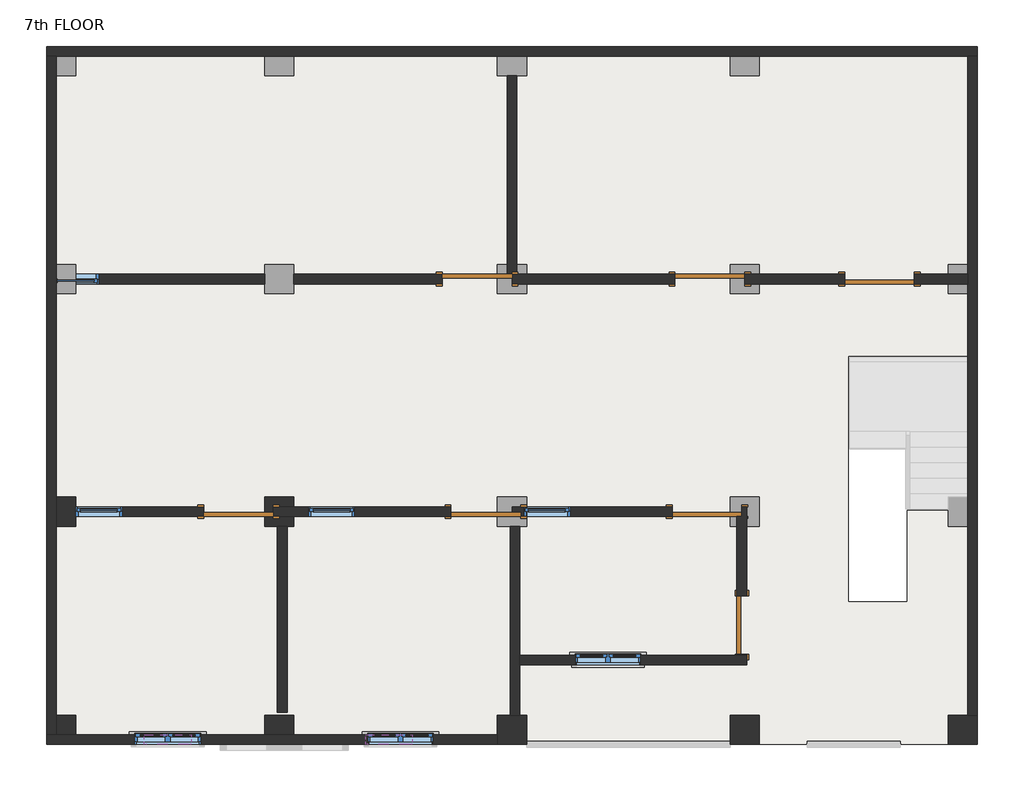
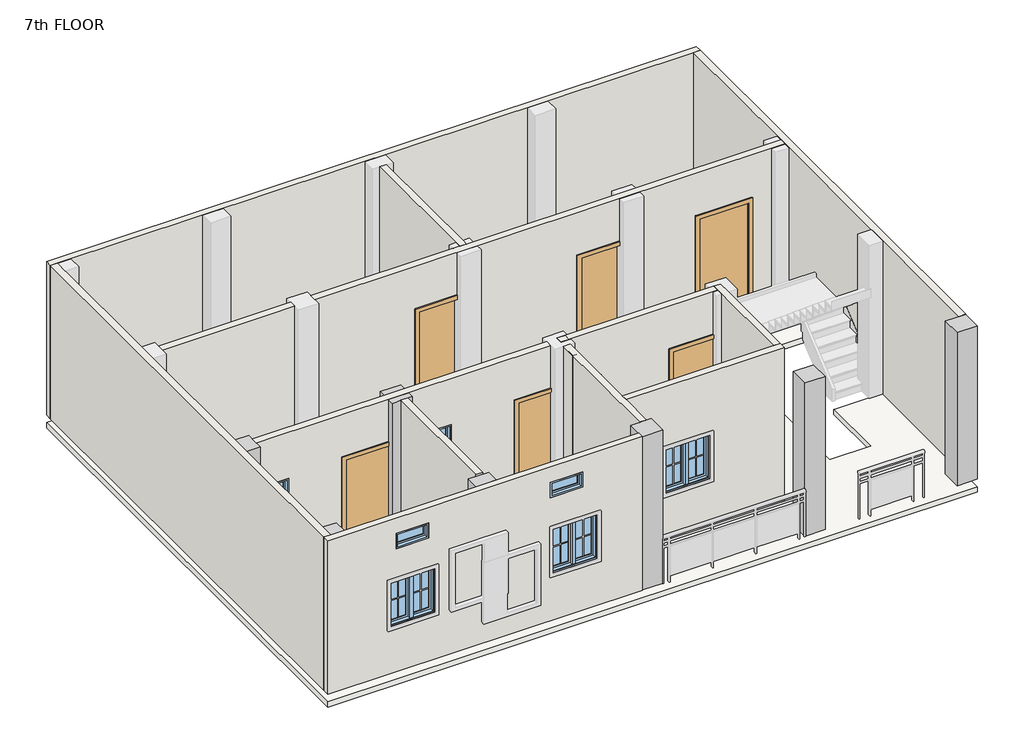
# One storey, part 1 of 2: 15 walls, 9 windows, 7 columns, 7 doors, 1 slab.
"""IFC4 building model written with IfcOpenShell, lengths in millimetres."""

from ifc_helpers import new_model, si_unit, frame, origin, place, context, project, spatial, polyline, outline, extrude, faceted_brep, transform, mapped, element, save
from components import door_e00f436c, door_a1797ceb, window_4c2727af, window_0bf3737e, window_78893e6c, window_0d9958e7

model = new_model("IFC4")

# Units and contexts
model_context = context("Model", 3, world=origin())
ifc_project = project(units=[si_unit("LENGTHUNIT", "METRE", prefix="MILLI")], contexts=[model_context])

# Site, building, storey
site = spatial("IfcSite", under=ifc_project)
building = spatial("IfcBuilding", under=site)
storey = spatial("IfcBuildingStorey", under=building, Name="7th FLOOR", Elevation=21183.6)

# Columns
placement = place(None, origin())
element("IfcColumn", 1, ObjectType="column family : column family", at=placement, inside=storey, context=model_context, shape_type="Brep", body=[
    faceted_brep([(-12576.097125, 2486.2065522, 21188.6), (-12957.097125, 2486.2065522, 21188.6), (-12957.097125, 2867.2065522, 21188.6), (-12576.097125, 2867.2065522, 21188.6), (-12576.097125, 2740.2065522, 21188.6), (-12842.797125, 2740.2065522, 21188.6), (-12842.797125, 2613.2065522, 21188.6), (-12576.097125, 2613.2065522, 21188.6), (-12576.097125, 2486.2065522, 24226.6), (-12576.097125, 2613.2065522, 24226.6), (-12957.097125, 2486.2065522, 24226.6), (-12957.097125, 2613.2065522, 24226.6), (-12957.097125, 2613.2065522, 23317.2), (-12957.097125, 2740.2065522, 23317.2), (-12957.097125, 2740.2065522, 24226.6), (-12957.097125, 2867.2065522, 24226.6), (-12576.097125, 2867.2065522, 24226.6), (-12842.797125, 2613.2065522, 23317.2), (-12842.797125, 2740.2065522, 23317.2), (-12576.097125, 2740.2065522, 24226.6)], [[[0, 1, 2, 3, 4, 5, 6, 7]], [[8, 0, 7, 9]], [[1, 0, 8, 10]], [[2, 1, 10, 11, 12, 13, 14, 15]], [[3, 2, 15, 16]], [[10, 8, 9, 11]], [[6, 17, 12, 11, 9, 7]], [[13, 18, 5, 4, 19, 14]], [[3, 16, 19, 4]], [[16, 15, 14, 19]], [[17, 18, 13, 12]], [[18, 17, 6, 5]]]),
])
element("IfcColumn", 2, ObjectType="column family : column family", at=placement, inside=storey, context=model_context, shape_type="SweptSolid", body=[
    extrude(outline(polyline([(-15433.597125, 2867.2065522), (-15433.597125, 2486.2065522), (-15687.597125, 2486.2065522), (-15687.597125, 2867.2065522), (-15433.597125, 2867.2065522)])), frame((0.0, 0.0, 21188.6), z_axis=(0.0, 0.0, 1.0), x_axis=(1.0, 0.0, 0.0)), (0.0, 0.0, 1.0), 3038.0),
])
element("IfcColumn", 3, ObjectType="column family : column family", at=placement, inside=storey, context=model_context, shape_type="SweptSolid", body=[
    extrude(outline(polyline([(-15433.597125, 9.7065522), (-15433.597125, -244.2934478), (-15687.597125, -244.2934478), (-15687.597125, 9.7065522), (-15433.597125, 9.7065522)])), frame((0.0, 0.0, 21188.6), z_axis=(0.0, 0.0, 1.0), x_axis=(1.0, 0.0, 0.0)), (0.0, 0.0, 1.0), 3038.0),
])
element("IfcColumn", 4, ObjectType="column family : column family", at=placement, inside=storey, context=model_context, shape_type="SweptSolid", body=[
    extrude(outline(polyline([(-3622.597125, 9.7065522), (-3622.597125, -371.2934478), (-4003.597125, -371.2934478), (-4003.597125, 9.7065522), (-3622.597125, 9.7065522)])), frame((0.0, 0.0, 21188.6), z_axis=(0.0, 0.0, 1.0), x_axis=(1.0, 0.0, 0.0)), (0.0, 0.0, 1.0), 3038.0),
])
element("IfcColumn", 5, ObjectType="column family : column family", at=placement, inside=storey, context=model_context, shape_type="SweptSolid", body=[
    extrude(outline(polyline([(-6480.097125, 9.7065522), (-6480.097125, -371.2934478), (-6861.097125, -371.2934478), (-6861.097125, 9.7065522), (-6480.097125, 9.7065522)])), frame((0.0, 0.0, 21188.6), z_axis=(0.0, 0.0, 1.0), x_axis=(1.0, 0.0, 0.0)), (0.0, 0.0, 1.0), 3038.0),
])
element("IfcColumn", 6, ObjectType="column family : column family", at=placement, inside=storey, context=model_context, shape_type="SweptSolid", body=[
    extrude(outline(polyline([(-9528.097125, 9.7065522), (-9528.097125, -371.2934478), (-9909.097125, -371.2934478), (-9909.097125, 9.7065522), (-9528.097125, 9.7065522)])), frame((0.0, 0.0, 21188.6), z_axis=(0.0, 0.0, 1.0), x_axis=(1.0, 0.0, 0.0)), (0.0, 0.0, 1.0), 3038.0),
])
element("IfcColumn", 7, ObjectType="column family : column family", at=placement, inside=storey, context=model_context, shape_type="SweptSolid", body=[
    extrude(outline(polyline([(-12957.097125, 9.7065522), (-12576.097125, 9.7065522), (-12576.097125, -244.2934478), (-12957.097125, -244.2934478), (-12957.097125, 9.7065522)])), frame((0.0, 0.0, 21188.6), z_axis=(0.0, 0.0, 1.0), x_axis=(1.0, 0.0, 0.0)), (0.0, 0.0, 1.0), 3038.0),
])

# Doors
door_shape = door_e00f436c(model_context)
element("IfcDoor", 8, ObjectType="Single-Flush : 30\" x 80\"", at=placement, inside=storey, context=model_context, shape_type="MappedRepresentation", body=[
    mapped(door_shape, transform((-6708.697125, 1190.8065522, 21183.6), x_axis=(0.0, -1.0, 0.0), y_axis=(1.0, 0.0, 0.0), z_axis=(0.0, 0.0, 1.0))),
])
door_2_shape = door_a1797ceb(model_context)
element("IfcDoor", 9, ObjectType="Single-Flush : 36\" x 84\"", at=placement, inside=storey, context=model_context, shape_type="MappedRepresentation", body=[
    mapped(door_2_shape, transform((-10175.797125, 5724.7065522, 21183.6), x_axis=(1.0, 0.0, 0.0), y_axis=(0.0, 1.0, 0.0), z_axis=(0.0, 0.0, 1.0))),
])
element("IfcDoor", 10, ObjectType="Single-Flush : 36\" x 84\"", at=placement, inside=storey, context=model_context, shape_type="MappedRepresentation", body=[
    mapped(door_2_shape, transform((-10061.497125, 2676.7065522, 21183.6), x_axis=(-1.0, 0.0, 0.0), y_axis=(0.0, -1.0, 0.0), z_axis=(0.0, 0.0, 1.0))),
])
element("IfcDoor", 11, ObjectType="Single-Flush : 36\" x 84\"", at=placement, inside=storey, context=model_context, shape_type="MappedRepresentation", body=[
    mapped(door_2_shape, transform((-13299.997125, 2676.7065522, 21183.6), x_axis=(-1.0, 0.0, 0.0), y_axis=(0.0, -1.0, 0.0), z_axis=(0.0, 0.0, 1.0))),
])
element("IfcDoor", 12, ObjectType="Single-Flush : 36\" x 84\"", at=placement, inside=storey, context=model_context, shape_type="MappedRepresentation", body=[
    mapped(door_2_shape, transform((-7127.797125, 5724.7065522, 21183.6), x_axis=(1.0, 0.0, 0.0), y_axis=(0.0, 1.0, 0.0), z_axis=(0.0, 0.0, 1.0))),
])
element("IfcDoor", 13, ObjectType="Single-Flush : 36\" x 84\"", at=placement, inside=storey, context=model_context, shape_type="MappedRepresentation", body=[
    mapped(door_2_shape, transform((-7165.897125, 2676.7065522, 21183.6), x_axis=(-1.0, 0.0, 0.0), y_axis=(0.0, -1.0, 0.0), z_axis=(0.0, 0.0, 1.0))),
])
element("IfcDoor", 14, ObjectType="Single-Flush : 36\" x 84\"", at=placement, inside=storey, context=model_context, shape_type="MappedRepresentation", body=[
    mapped(door_2_shape, transform((-4905.297125, 5724.7065522, 21183.6), x_axis=(-1.0, 0.0, 0.0), y_axis=(0.0, -1.0, 0.0), z_axis=(0.0, 0.0, 1.0))),
])

# Slab
element("IfcSlab", 15, ObjectType="Generic - 4\"", at=placement, inside=storey, context=model_context, shape_type="SweptSolid", body=[
    extrude(outline(polyline([(-3622.597125, 8772.7065522), (-3622.597125, -371.2934478), (-15814.597125, -371.2934478), (-15814.597125, 8772.7065522), (-3622.597125, 8772.7065522)]), holes=[polyline([(-3734.357125, 4711.0719226), (-5310.2646464, 4711.0719226), (-5310.2646464, 1502.3126957), (-4547.7736682, 1502.3126957), (-4547.7736682, 2699.911213), (-3734.357125, 2699.911213), (-3734.357125, 4711.0719226)])]), frame((0.0, 0.0, 20929.6), z_axis=(0.0, 0.0, 1.0), x_axis=(1.0, 0.0, 0.0)), (0.0, 0.0, 1.0), 101.6),
])

# Walls
element("IfcWall", 16, ObjectType="Generic - 5\"", at=placement, inside=storey, context=model_context, shape_type="Brep", body=[
    faceted_brep([(-15814.597125, 8645.7065522, 21183.6), (-15687.597125, 8645.7065522, 21183.6), (-3749.597125, 8645.7065522, 21183.6), (-3622.597125, 8645.7065522, 21183.6), (-3622.597125, 8645.7065522, 24231.6), (-3749.597125, 8645.7065522, 24231.6), (-15687.597125, 8645.7065522, 24231.6), (-15814.597125, 8645.7065522, 24231.6), (-15814.597125, 8772.7065522, 21183.6), (-15814.597125, 8772.7065522, 24231.6), (-3622.597125, 8772.7065522, 24231.6), (-3622.597125, 8772.7065522, 21183.6)], [[[0, 1, 2, 3, 4, 5, 6, 7]], [[8, 9, 10, 11]], [[3, 2, 1, 0, 8, 11]], [[7, 6, 5, 4, 10, 9]], [[4, 3, 11, 10]], [[0, 7, 9, 8]]]),
])
element("IfcWall", 17, ObjectType="Generic - 5\"", at=placement, inside=storey, context=model_context, shape_type="Brep", body=[
    faceted_brep([(-3749.597125, 8645.7065522, 21183.6), (-3749.597125, 5788.2065522, 21183.6), (-3749.597125, 5661.2065522, 21183.6), (-3749.597125, 9.7065522, 21183.6), (-3749.597125, 9.7065522, 24231.6), (-3749.597125, 5661.2065522, 24231.6), (-3749.597125, 5788.2065522, 24231.6), (-3749.597125, 8645.7065522, 24231.6), (-3622.597125, 8645.7065522, 21183.6), (-3622.597125, 8645.7065522, 24231.6), (-3622.597125, 9.7065522, 24231.6), (-3622.597125, 9.7065522, 24226.6), (-3622.597125, 9.7065522, 21188.6), (-3622.597125, 9.7065522, 21183.6)], [[[0, 1, 2, 3, 4, 5, 6, 7]], [[8, 9, 10, 11, 12, 13]], [[3, 2, 1, 0, 8, 13]], [[4, 3, 13, 12, 11, 10]], [[7, 6, 5, 4, 10, 9]], [[0, 7, 9, 8]]]),
])
element("IfcWall", 18, ObjectType="Generic - 5\"", at=placement, inside=storey, context=model_context, shape_type="Brep", body=[
    faceted_brep([(-9909.097125, -244.2934478, 21183.6), (-15687.597125, -244.2934478, 21183.6), (-15814.597125, -244.2934478, 21183.6), (-15814.597125, -244.2934478, 24231.6), (-15687.597125, -244.2934478, 24231.6), (-9909.097125, -244.2934478, 24231.6), (-13795.297125, -244.2934478, 23012.4), (-14658.897125, -244.2934478, 23012.4), (-14658.897125, -244.2934478, 22098.0), (-13795.297125, -244.2934478, 22098.0), (-10747.297125, -244.2934478, 23012.4), (-11610.897125, -244.2934478, 23012.4), (-11610.897125, -244.2934478, 22098.0), (-10747.297125, -244.2934478, 22098.0), (-13922.297125, -244.2934478, 23926.8), (-14531.897125, -244.2934478, 23926.8), (-14531.897125, -244.2934478, 23622.0), (-13922.297125, -244.2934478, 23622.0), (-11026.697125, -244.2934478, 23926.8), (-11636.297125, -244.2934478, 23926.8), (-11636.297125, -244.2934478, 23622.0), (-11026.697125, -244.2934478, 23622.0), (-9909.097125, -371.2934478, 21183.6), (-9909.097125, -371.2934478, 21188.6), (-9909.097125, -371.2934478, 24226.6), (-9909.097125, -371.2934478, 24231.6), (-15814.597125, -371.2934478, 24231.6), (-15814.597125, -371.2934478, 21183.6), (-13795.297125, -371.2934478, 23012.4), (-13795.297125, -371.2934478, 22098.0), (-14658.897125, -371.2934478, 22098.0), (-14658.897125, -371.2934478, 23012.4), (-10747.297125, -371.2934478, 23012.4), (-10747.297125, -371.2934478, 22098.0), (-11610.897125, -371.2934478, 22098.0), (-11610.897125, -371.2934478, 23012.4), (-13922.297125, -371.2934478, 23926.8), (-13922.297125, -371.2934478, 23622.0), (-14531.897125, -371.2934478, 23622.0), (-14531.897125, -371.2934478, 23926.8), (-11026.697125, -371.2934478, 23926.8), (-11026.697125, -371.2934478, 23622.0), (-11636.297125, -371.2934478, 23622.0), (-11636.297125, -371.2934478, 23926.8)], [[[0, 1, 2, 3, 4, 5], [6, 7, 8, 9], [10, 11, 12, 13], [14, 15, 16, 17], [18, 19, 20, 21]], [[22, 23, 24, 25, 26, 27], [28, 29, 30, 31], [32, 33, 34, 35], [36, 37, 38, 39], [40, 41, 42, 43]], [[2, 1, 0, 22, 27]], [[5, 4, 3, 26, 25]], [[0, 5, 25, 24, 23, 22]], [[3, 2, 27, 26]], [[29, 28, 6, 9]], [[30, 29, 9, 8]], [[31, 30, 8, 7]], [[28, 31, 7, 6]], [[33, 32, 10, 13]], [[34, 33, 13, 12]], [[35, 34, 12, 11]], [[32, 35, 11, 10]], [[37, 36, 14, 17]], [[38, 37, 17, 16]], [[39, 38, 16, 15]], [[36, 39, 15, 14]], [[41, 40, 18, 21]], [[42, 41, 21, 20]], [[43, 42, 20, 19]], [[40, 43, 19, 18]]]),
])
element("IfcWall", 19, ObjectType="Generic - 5\"", at=placement, inside=storey, context=model_context, shape_type="Brep", body=[
    faceted_brep([(-15687.597125, -244.2934478, 21183.6), (-15687.597125, 8645.7065522, 21183.6), (-15687.597125, 8645.7065522, 21188.6), (-15687.597125, 8645.7065522, 24226.6), (-15687.597125, 8645.7065522, 24231.6), (-15687.597125, -244.2934478, 24231.6), (-15687.597125, -244.2934478, 24226.6), (-15687.597125, -244.2934478, 21188.6), (-15814.597125, -244.2934478, 21183.6), (-15814.597125, -244.2934478, 24231.6), (-15814.597125, 8645.7065522, 24231.6), (-15814.597125, 8645.7065522, 21183.6)], [[[0, 1, 2, 3, 4, 5, 6, 7]], [[8, 9, 10, 11]], [[1, 0, 8, 11]], [[5, 4, 10, 9]], [[4, 3, 2, 1, 11, 10]], [[0, 7, 6, 5, 9, 8]]]),
])
element("IfcWall", 20, ObjectType="Generic - 5\"", at=placement, inside=storey, context=model_context, shape_type="SweptSolid", body=[
    extrude(outline(polyline([(21183.6, -15433.597125), (21183.6, -12957.097125), (24231.6, -12957.097125), (24231.6, -15433.597125), (23317.2, -15433.597125), (23317.2, -15128.797125), (21488.4, -15128.797125), (21488.4, -15433.597125), (21183.6, -15433.597125)])), frame((0.0, 5661.2065522, 0.0), z_axis=(0.0, 1.0, 0.0), x_axis=(0.0, 0.0, 1.0)), (0.0, 0.0, 1.0), 127.0),
])
element("IfcWall", 21, ObjectType="Generic - 5\"", at=placement, inside=storey, context=model_context, shape_type="Brep", body=[
    faceted_brep([(-9782.097125, 8391.7065522, 21183.6), (-9782.097125, 5788.2065522, 21183.6), (-9782.097125, 5788.2065522, 21188.6), (-9782.097125, 5788.2065522, 23317.2), (-9782.097125, 5788.2065522, 24226.6), (-9782.097125, 5788.2065522, 24231.6), (-9782.097125, 8391.7065522, 24231.6), (-9655.097125, 8391.7065522, 21183.6), (-9655.097125, 8391.7065522, 24231.6), (-9655.097125, 5788.2065522, 24231.6), (-9655.097125, 5788.2065522, 24226.6), (-9655.097125, 5788.2065522, 21188.6), (-9655.097125, 5788.2065522, 21183.6), (-9718.597125, 5788.2065522, 21183.6)], [[[0, 1, 2, 3, 4, 5, 6]], [[7, 8, 9, 10, 11, 12]], [[1, 0, 7, 12, 13]], [[6, 5, 9, 8]], [[0, 6, 8, 7]], [[5, 4, 3, 2, 1, 13, 12, 11, 10, 9]]]),
])
element("IfcWall", 22, ObjectType="Generic - 5\"", at=placement, inside=storey, context=model_context, shape_type="Brep", body=[
    faceted_brep([(-6670.597125, 5661.2065522, 21183.6), (-5362.497125, 5661.2065522, 21183.6), (-5362.497125, 5661.2065522, 23317.2), (-4448.097125, 5661.2065522, 23317.2), (-4448.097125, 5661.2065522, 21183.6), (-3749.597125, 5661.2065522, 21183.6), (-3749.597125, 5661.2065522, 21188.6), (-3749.597125, 5661.2065522, 24226.6), (-3749.597125, 5661.2065522, 24231.6), (-12576.097125, 5661.2065522, 24231.6), (-12576.097125, 5661.2065522, 21183.6), (-10632.997125, 5661.2065522, 21183.6), (-10632.997125, 5661.2065522, 23317.2), (-9909.097125, 5661.2065522, 23317.2), (-9718.597125, 5661.2065522, 23317.2), (-9718.597125, 5661.2065522, 21188.6), (-9718.597125, 5661.2065522, 21183.6), (-7584.997125, 5661.2065522, 21183.6), (-7584.997125, 5661.2065522, 23317.2), (-6861.097125, 5661.2065522, 23317.2), (-6670.597125, 5661.2065522, 23317.2), (-6670.597125, 5661.2065522, 21188.6), (-5362.497125, 5788.2065522, 23317.2), (-5362.497125, 5788.2065522, 21183.6), (-6670.597125, 5788.2065522, 21183.6), (-6670.597125, 5788.2065522, 21188.6), (-6670.597125, 5788.2065522, 23317.2), (-6861.097125, 5788.2065522, 23317.2), (-7584.997125, 5788.2065522, 23317.2), (-7584.997125, 5788.2065522, 21183.6), (-9655.097125, 5788.2065522, 21183.6), (-9718.597125, 5788.2065522, 21183.6), (-9718.597125, 5788.2065522, 21188.6), (-9718.597125, 5788.2065522, 23317.2), (-9782.097125, 5788.2065522, 23317.2), (-9909.097125, 5788.2065522, 23317.2), (-10632.997125, 5788.2065522, 23317.2), (-10632.997125, 5788.2065522, 21183.6), (-12576.097125, 5788.2065522, 21183.6), (-12576.097125, 5788.2065522, 24231.6), (-9782.097125, 5788.2065522, 24231.6), (-9655.097125, 5788.2065522, 24231.6), (-3749.597125, 5788.2065522, 24231.6), (-3749.597125, 5788.2065522, 24226.6), (-3749.597125, 5788.2065522, 21188.6), (-3749.597125, 5788.2065522, 21183.6), (-4448.097125, 5788.2065522, 21183.6), (-4448.097125, 5788.2065522, 23317.2)], [[[0, 1, 2, 3, 4, 5, 6, 7, 8, 9, 10, 11, 12, 13, 14, 15, 16, 17, 18, 19, 20, 21]], [[22, 23, 24, 25, 26, 27, 28, 29, 30, 31, 32, 33, 34, 35, 36, 37, 38, 39, 40, 41, 42, 43, 44, 45, 46, 47]], [[11, 10, 38, 37]], [[17, 16, 31, 30, 29]], [[46, 45, 5, 4]], [[24, 23, 1, 0]], [[9, 8, 42, 41, 40, 39]], [[10, 9, 39, 38]], [[8, 7, 6, 5, 45, 44, 43, 42]], [[33, 32, 31, 16, 15, 14]], [[36, 35, 34, 33, 14, 13, 12]], [[37, 36, 12, 11]], [[26, 25, 24, 0, 21, 20]], [[28, 27, 26, 20, 19, 18]], [[29, 28, 18, 17]], [[2, 1, 23, 22]], [[3, 2, 22, 47]], [[4, 3, 47, 46]]]),
])
element("IfcWall", 23, ObjectType="Generic - 5\"", at=placement, inside=storey, context=model_context, shape_type="Brep", body=[
    faceted_brep([(-14823.997125, 2613.2065522, 21488.4), (-15433.597125, 2613.2065522, 21488.4), (-15433.597125, 2613.2065522, 21183.6), (-13757.197125, 2613.2065522, 21183.6), (-13757.197125, 2613.2065522, 23317.2), (-12957.097125, 2613.2065522, 23317.2), (-12842.797125, 2613.2065522, 23317.2), (-12842.797125, 2613.2065522, 21188.6), (-12842.797125, 2613.2065522, 21183.6), (-10518.697125, 2613.2065522, 21183.6), (-10518.697125, 2613.2065522, 23317.2), (-9909.097125, 2613.2065522, 23317.2), (-9909.097125, 2613.2065522, 24231.6), (-15433.597125, 2613.2065522, 24231.6), (-15433.597125, 2613.2065522, 23317.2), (-14823.997125, 2613.2065522, 23317.2), (-12385.597125, 2613.2065522, 23317.2), (-11775.997125, 2613.2065522, 23317.2), (-11775.997125, 2613.2065522, 21488.4), (-12385.597125, 2613.2065522, 21488.4), (-15433.597125, 2740.2065522, 21183.6), (-15433.597125, 2740.2065522, 21488.4), (-14823.997125, 2740.2065522, 21488.4), (-14823.997125, 2740.2065522, 23317.2), (-15433.597125, 2740.2065522, 23317.2), (-15433.597125, 2740.2065522, 24231.6), (-9909.097125, 2740.2065522, 24231.6), (-9909.097125, 2740.2065522, 23317.2), (-10518.697125, 2740.2065522, 23317.2), (-10518.697125, 2740.2065522, 21183.6), (-12842.797125, 2740.2065522, 21183.6), (-12842.797125, 2740.2065522, 21188.6), (-12842.797125, 2740.2065522, 23317.2), (-12957.097125, 2740.2065522, 23317.2), (-13757.197125, 2740.2065522, 23317.2), (-13757.197125, 2740.2065522, 21183.6), (-12385.597125, 2740.2065522, 23317.2), (-12385.597125, 2740.2065522, 21488.4), (-11775.997125, 2740.2065522, 21488.4), (-11775.997125, 2740.2065522, 23317.2)], [[[0, 1, 2, 3, 4, 5, 6, 7, 8, 9, 10, 11, 12, 13, 14, 15], [16, 17, 18, 19]], [[20, 21, 22, 23, 24, 25, 26, 27, 28, 29, 30, 31, 32, 33, 34, 35], [36, 37, 38, 39]], [[30, 29, 9, 8]], [[20, 35, 3, 2]], [[26, 12, 11, 27]], [[13, 12, 26, 25]], [[14, 13, 25, 24]], [[2, 1, 21, 20]], [[28, 10, 9, 29]], [[10, 28, 27, 11]], [[4, 3, 35, 34]], [[6, 5, 4, 34, 33, 32]], [[8, 7, 6, 32, 31, 30]], [[22, 21, 1, 0]], [[23, 22, 0, 15]], [[24, 23, 15, 14]], [[37, 36, 16, 19]], [[38, 37, 19, 18]], [[39, 38, 18, 17]], [[36, 39, 17, 16]]]),
])
element("IfcWall", 24, ObjectType="Generic - 5\"", at=placement, inside=storey, context=model_context, shape_type="Brep", body=[
    faceted_brep([(-9616.997125, 9.7065522, 21183.6), (-9616.997125, 670.1065522, 21183.6), (-9616.997125, 797.1065522, 21183.6), (-9616.997125, 2486.2065522, 21183.6), (-9616.997125, 2486.2065522, 24231.6), (-9616.997125, 797.1065522, 24231.6), (-9616.997125, 670.1065522, 24231.6), (-9616.997125, 9.7065522, 24231.6), (-9743.997125, 9.7065522, 21183.6), (-9743.997125, 9.7065522, 24231.6), (-9743.997125, 2486.2065522, 24231.6), (-9743.997125, 2486.2065522, 21183.6)], [[[0, 1, 2, 3, 4, 5, 6, 7]], [[8, 9, 10, 11]], [[3, 2, 1, 0, 8, 11]], [[4, 3, 11, 10]], [[7, 6, 5, 4, 10, 9]], [[0, 7, 9, 8]]]),
])
element("IfcWall", 25, ObjectType="Generic - 5\"", at=placement, inside=storey, context=model_context, shape_type="SweptSolid", body=[
    extrude(outline(polyline([(-9743.997125, 2181.4065522), (-9743.997125, 2486.2065522), (-9616.997125, 2486.2065522), (-9616.997125, 2181.4065522), (-9743.997125, 2181.4065522)])), frame((0.0, 0.0, 21183.6), z_axis=(0.0, 0.0, 1.0), x_axis=(1.0, 0.0, 0.0)), (0.0, 0.0, 1.0), 3048.0),
])
element("IfcWall", 26, ObjectType="Generic - 5\"", at=placement, inside=storey, context=model_context, shape_type="Brep", body=[
    faceted_brep([(-6772.197125, 2613.2065522, 24231.6), (-9718.597125, 2613.2065522, 24231.6), (-9718.597125, 2613.2065522, 24226.6), (-9718.597125, 2613.2065522, 21188.6), (-9718.597125, 2613.2065522, 21183.6), (-7623.097125, 2613.2065522, 21183.6), (-7623.097125, 2613.2065522, 23317.2), (-6861.097125, 2613.2065522, 23317.2), (-6772.197125, 2613.2065522, 23317.2), (-6772.197125, 2613.2065522, 24226.6), (-9566.197125, 2613.2065522, 23317.2), (-9528.097125, 2613.2065522, 23317.2), (-8956.597125, 2613.2065522, 23317.2), (-8956.597125, 2613.2065522, 21488.4), (-9528.097125, 2613.2065522, 21488.4), (-9566.197125, 2613.2065522, 21488.4), (-9718.597125, 2740.2065522, 24231.6), (-6772.197125, 2740.2065522, 24231.6), (-6772.197125, 2740.2065522, 23317.2), (-6861.097125, 2740.2065522, 23317.2), (-7623.097125, 2740.2065522, 23317.2), (-7623.097125, 2740.2065522, 21183.6), (-9718.597125, 2740.2065522, 21183.6), (-9718.597125, 2740.2065522, 21188.6), (-9718.597125, 2740.2065522, 24226.6), (-9566.197125, 2740.2065522, 23317.2), (-9566.197125, 2740.2065522, 21488.4), (-9528.097125, 2740.2065522, 21488.4), (-8956.597125, 2740.2065522, 21488.4), (-8956.597125, 2740.2065522, 23317.2), (-9528.097125, 2740.2065522, 23317.2)], [[[0, 1, 2, 3, 4, 5, 6, 7, 8, 9], [10, 11, 12, 13, 14, 15]], [[16, 17, 18, 19, 20, 21, 22, 23, 24], [25, 26, 27, 28, 29, 30]], [[4, 22, 21, 5]], [[1, 0, 17, 16]], [[4, 3, 2, 1, 16, 24, 23, 22]], [[26, 25, 10, 15]], [[28, 27, 26, 15, 14, 13]], [[29, 28, 13, 12]], [[25, 30, 29, 12, 11, 10]], [[20, 6, 5, 21]], [[6, 20, 19, 18, 8, 7]], [[17, 0, 9, 8, 18]]]),
])
element("IfcWall", 27, ObjectType="Generic - 5\"", at=placement, inside=storey, context=model_context, shape_type="Brep", body=[
    faceted_brep([(-6645.197125, 797.1065522, 21183.6), (-6645.197125, 809.8065522, 21183.6), (-6645.197125, 809.8065522, 23215.6), (-6645.197125, 1571.8065522, 23215.6), (-6645.197125, 1571.8065522, 21183.6), (-6645.197125, 2740.2065522, 21183.6), (-6645.197125, 2740.2065522, 21188.6), (-6645.197125, 2740.2065522, 24226.6), (-6645.197125, 2740.2065522, 24231.6), (-6645.197125, 797.1065522, 24231.6), (-6772.197125, 809.8065522, 23215.6), (-6772.197125, 809.8065522, 21183.6), (-6772.197125, 797.1065522, 21183.6), (-6772.197125, 797.1065522, 24231.6), (-6772.197125, 2613.2065522, 24231.6), (-6772.197125, 2740.2065522, 24231.6), (-6772.197125, 2740.2065522, 23317.2), (-6772.197125, 2613.2065522, 23317.2), (-6772.197125, 2613.2065522, 21188.6), (-6772.197125, 2613.2065522, 21183.6), (-6772.197125, 1571.8065522, 21183.6), (-6772.197125, 1571.8065522, 23215.6), (-6708.697125, 2613.2065522, 21183.6), (-6708.697125, 2740.2065522, 21183.6), (-6708.697125, 2613.2065522, 23317.2), (-6708.697125, 2613.2065522, 21188.6), (-6708.697125, 2740.2065522, 23317.2), (-6708.697125, 2740.2065522, 21188.6)], [[[0, 1, 2, 3, 4, 5, 6, 7, 8, 9]], [[10, 11, 12, 13, 14, 15, 16, 17, 18, 19, 20, 21]], [[20, 19, 22, 23, 5, 4]], [[12, 11, 1, 0]], [[9, 8, 15, 14, 13]], [[24, 25, 22, 19, 18, 17]], [[26, 24, 17, 16]], [[22, 25, 24, 26, 27, 23]], [[8, 7, 6, 5, 23, 27, 26, 16, 15]], [[0, 9, 13, 12]], [[2, 1, 11, 10]], [[3, 2, 10, 21]], [[4, 3, 21, 20]]]),
])
element("IfcWall", 28, ObjectType="Generic - 5\"", at=placement, inside=storey, context=model_context, shape_type="Brep", body=[
    faceted_brep([(-9718.597125, 2613.2065522, 21183.6), (-9566.197125, 2613.2065522, 21183.6), (-9566.197125, 2613.2065522, 21488.4), (-9566.197125, 2613.2065522, 23317.2), (-9566.197125, 2613.2065522, 24231.6), (-9718.597125, 2613.2065522, 24231.6), (-9718.597125, 2613.2065522, 24226.6), (-9718.597125, 2613.2065522, 21188.6), (-9718.597125, 2740.2065522, 21183.6), (-9718.597125, 2740.2065522, 21188.6), (-9718.597125, 2740.2065522, 24226.6), (-9718.597125, 2740.2065522, 24231.6), (-9566.197125, 2740.2065522, 24231.6), (-9566.197125, 2740.2065522, 23317.2), (-9566.197125, 2740.2065522, 21488.4), (-9566.197125, 2740.2065522, 21183.6)], [[[0, 1, 2, 3, 4, 5, 6, 7]], [[8, 9, 10, 11, 12, 13, 14, 15]], [[1, 0, 8, 15]], [[4, 3, 2, 1, 15, 14, 13, 12]], [[5, 4, 12, 11]], [[0, 7, 6, 5, 11, 10, 9, 8]]]),
])
element("IfcWall", 29, ObjectType="Generic - 5\"", at=placement, inside=storey, context=model_context, shape_type="SweptSolid", body=[
    extrude(outline(polyline([(-12791.997125, 47.8065522), (-12791.997125, 2486.2065522), (-12664.997125, 2486.2065522), (-12664.997125, 47.8065522), (-12791.997125, 47.8065522)])), frame((0.0, 0.0, 21183.6), z_axis=(0.0, 0.0, 1.0), x_axis=(1.0, 0.0, 0.0)), (0.0, 0.0, 1.0), 3048.0),
])
element("IfcWall", 30, ObjectType="Generic - 5\"", at=placement, inside=storey, context=model_context, shape_type="Brep", body=[
    faceted_brep([(-9616.997125, 670.1065522, 21183.6), (-6645.197125, 670.1065522, 21183.6), (-6645.197125, 670.1065522, 24231.6), (-9616.997125, 670.1065522, 24231.6), (-8029.497125, 670.1065522, 23012.4), (-8029.497125, 670.1065522, 22098.0), (-8893.097125, 670.1065522, 22098.0), (-8893.097125, 670.1065522, 23012.4), (-9616.997125, 797.1065522, 21183.6), (-9616.997125, 797.1065522, 24231.6), (-6772.197125, 797.1065522, 24231.6), (-6645.197125, 797.1065522, 24231.6), (-6645.197125, 797.1065522, 21183.6), (-6772.197125, 797.1065522, 21183.6), (-8029.497125, 797.1065522, 23012.4), (-8893.097125, 797.1065522, 23012.4), (-8893.097125, 797.1065522, 22098.0), (-8029.497125, 797.1065522, 22098.0)], [[[0, 1, 2, 3], [4, 5, 6, 7]], [[8, 9, 10, 11, 12, 13], [14, 15, 16, 17]], [[1, 0, 8, 13, 12]], [[3, 2, 11, 10, 9]], [[0, 3, 9, 8]], [[2, 1, 12, 11]], [[5, 4, 14, 17]], [[6, 5, 17, 16]], [[7, 6, 16, 15]], [[4, 7, 15, 14]]]),
])

# Windows
window_shape = window_4c2727af(model_context)
element("IfcWindow", 31, ObjectType="Fixed : 24\" x 12\"", at=placement, inside=storey, context=model_context, shape_type="MappedRepresentation", body=[
    mapped(window_shape, transform((-14188.997125, -307.7934478, 22707.6), x_axis=(1.0, 0.0, 0.0), y_axis=(0.0, 1.0, 0.0), z_axis=(0.0, 0.0, 1.0))),
])
element("IfcWindow", 32, ObjectType="Fixed : 24\" x 12\"", at=placement, inside=storey, context=model_context, shape_type="MappedRepresentation", body=[
    mapped(window_shape, transform((-11293.397125, -307.7934478, 22707.6), x_axis=(1.0, 0.0, 0.0), y_axis=(0.0, 1.0, 0.0), z_axis=(0.0, 0.0, 1.0))),
])
window_2_shape = window_0bf3737e(model_context)
element("IfcWindow", 33, ObjectType="Fixed : 24\" x 72\"", at=placement, inside=storey, context=model_context, shape_type="MappedRepresentation", body=[
    mapped(window_2_shape, transform((-15471.697125, 5724.7065522, 21183.6), x_axis=(-1.0, 0.0, 0.0), y_axis=(0.0, -1.0, 0.0), z_axis=(0.0, 0.0, 1.0))),
])
window_3_shape = window_78893e6c(model_context)
element("IfcWindow", 34, ObjectType="Fixed : 24\" x 72\"", at=placement, inside=storey, context=model_context, shape_type="MappedRepresentation", body=[
    mapped(window_3_shape, transform((-15166.897125, 2676.7065522, 21183.6), x_axis=(-1.0, 0.0, 0.0), y_axis=(0.0, -1.0, 0.0), z_axis=(0.0, 0.0, 1.0))),
])
element("IfcWindow", 35, ObjectType="Fixed : 24\" x 72\"", at=placement, inside=storey, context=model_context, shape_type="MappedRepresentation", body=[
    mapped(window_3_shape, transform((-12118.897125, 2676.7065522, 21183.6), x_axis=(-1.0, 0.0, 0.0), y_axis=(0.0, -1.0, 0.0), z_axis=(0.0, 0.0, 1.0))),
])
element("IfcWindow", 36, ObjectType="Fixed : 24\" x 72\"", at=placement, inside=storey, context=model_context, shape_type="MappedRepresentation", body=[
    mapped(window_3_shape, transform((-9299.497125, 2676.7065522, 21183.6), x_axis=(-1.0, 0.0, 0.0), y_axis=(0.0, -1.0, 0.0), z_axis=(0.0, 0.0, 1.0))),
])
window_4_shape = window_0d9958e7(model_context)
element("IfcWindow", 37, ObjectType="Window-Casement-Double : 34\" x 36\"", at=placement, inside=storey, context=model_context, shape_type="MappedRepresentation", body=[
    mapped(window_4_shape, transform((-14227.097125, -307.7934478, 21183.6), x_axis=(1.0, 0.0, 0.0), y_axis=(0.0, 1.0, 0.0), z_axis=(0.0, 0.0, 1.0))),
])
element("IfcWindow", 38, ObjectType="Window-Casement-Double : 34\" x 36\"", at=placement, inside=storey, context=model_context, shape_type="MappedRepresentation", body=[
    mapped(window_4_shape, transform((-11179.097125, -307.7934478, 21183.6), x_axis=(1.0, 0.0, 0.0), y_axis=(0.0, 1.0, 0.0), z_axis=(0.0, 0.0, 1.0))),
])
element("IfcWindow", 39, ObjectType="Window-Casement-Double : 34\" x 36\"", at=placement, inside=storey, context=model_context, shape_type="MappedRepresentation", body=[
    mapped(window_4_shape, transform((-8461.297125, 733.6065522, 21183.6), x_axis=(1.0, 0.0, 0.0), y_axis=(0.0, 1.0, 0.0), z_axis=(0.0, 0.0, 1.0))),
])

save(model, "model.ifc")

# Revit data of these elements
# Type "column family : column family"
#   w2 [instance default] = 0' - 9.88189"
#   w1 [instance default] = 0' - 9.01575"
#   Depth = 1' - 11.62205"
#   Width = 1' - 11.62205"
# Type "Single-Flush : 30\" x 80\""
#   Type Mark = "5"
#   Construction Type Id = "MDOOR"
#   Assembly Code = "C1020"
#   Analytic Construction = "Metal"
#   Thickness = 0' - 2"
#   Heat Transfer Coefficient (U) = 0.651978 BTU/(h·ft²·°F)
#   Height = 6' - 8"
#   Trim Projection Ext = 0' - 1"
#   Trim Projection Int = 0' - 1"
#   Trim Width = 0' - 3"
#   Width = 2' - 6"
#   Define Thermal Properties by = 1
#   Define Thermal Properties by = 1
#   Door Material = Door - Panel
#   Frame Material = Door - Frame
#   Visual Light Transmittance = 0
#   Solar Heat Gain Coefficient = 0
#   Function = (empty or 0)
#   Wall Closure = (empty or 0)
# Type "Single-Flush : 36\" x 84\""
#   Type Mark = "1"
#   Construction Type Id = "MDOOR"
#   Assembly Code = "C1020"
#   Analytic Construction = "Metal"
#   Thickness = 0' - 2"
#   Heat Transfer Coefficient (U) = 0.651978 BTU/(h·ft²·°F)
#   Height = 7' - 0"
#   Trim Projection Ext = 0' - 1"
#   Trim Projection Int = 0' - 1"
#   Trim Width = 0' - 3"
#   Width = 3' - 0"
#   Define Thermal Properties by = 1
#   Define Thermal Properties by = 1
#   Door Material = Door - Panel
#   Frame Material = Door - Frame
#   Visual Light Transmittance = 0
#   Solar Heat Gain Coefficient = 0
#   Function = (empty or 0)
#   Wall Closure = (empty or 0)
# Type "Generic - 4\""
#   Assembly Code = "B1010"
#   Function = 0
#   Layers, outside or top first: 0' - 4" no material (function 1)
# Type "Generic - 5\""
#   Assembly Code = "B2010"
#   Layers, outside or top first: 0' - 5" no material (function 1)
# Type "Fixed : 24\" x 12\""
#   Type Mark = "4"
#   Construction Type Id = "GSP4R"
#   Assembly Code = "B2020100"
#   Analytic Construction = "1/8 in Pilkington single glazing"
#   Visual Light Transmittance = 0.9
#   Solar Heat Gain Coefficient = 0.78
#   Heat Transfer Coefficient (U) = 0.6496 BTU/(h·ft²·°F)
#   Height = 1' - 0"
#   Default Sill Height = 3' - 0"
#   Width = 2' - 0"
#   Window Inset = 0' - 0 3/4"
#   Define Thermal Properties by = 1
#   Define Thermal Properties by = 1
#   Glass Pane Material = Glass
#   Sash Material = Sash
#   Wall Closure = (empty or 0)
# Type "Fixed : 24\" x 72\""
#   Type Mark = "7"
#   Construction Type Id = "GSP4R"
#   Assembly Code = "B2020100"
#   Analytic Construction = "1/8 in Pilkington single glazing"
#   Visual Light Transmittance = 0.9
#   Solar Heat Gain Coefficient = 0.78
#   Heat Transfer Coefficient (U) = 0.6496 BTU/(h·ft²·°F)
#   Height = 6' - 0"
#   Default Sill Height = 1' - 0"
#   Width = 2' - 0"
#   Window Inset = 0' - 0 3/4"
#   Define Thermal Properties by = 1
#   Define Thermal Properties by = 1
#   Glass Pane Material = Glass
#   Sash Material = Sash
#   Wall Closure = (empty or 0)
# Type "Window-Casement-Double : 34\" x 36\""
#   Type Mark = "14"
#   Fire Rating = "0.5h"
#   Assembly Code = "B2020100"
#   Analytic Construction = "Double glazing - domestic"
#   Frame Extension [instance default] = 0' - 0 1/4"
#   Window Inset [instance default] = 0' - 0"
#   Wall Thickness [instance default] = 0' - 6"
#   Interior Wall Closure [instance default] = 0' - 2 1/4"
#   Half Width = 1' - 5"
#   Visual Light Transmittance = 0.81
#   Thermal Resistance (R) = 1.8146 (h·ft²·°F)/BTU
#   Solar Heat Gain Coefficient = 0.76
#   Rough Width = 2' - 10 1/2"
#   Rough Height = 3' - 0 1/2"
#   Height = 3' - 0"
#   Heat Transfer Coefficient (U) = 0.5511 BTU/(h·ft²·°F)
#   Exterior Wall Closure [instance default] = 0' - 1 1/4"
#   Extension Jamb [instance default] = 0' - 2 1/4"
#   Default Sill Height = 3' - 0"
#   Width = 2' - 10"
#   Define Thermal Properties by = 0
#   Muntin Visibility = yes
#   Interior Trim Visibility [instance default] = yes
#   Exterior Trim Visibility [instance default] = yes
#   Extension Jamb Visibility [instance default] = yes
#   Interior Trim Material = Wood - Stained
#   Muntin Pattern = Muntin Pattern_2x2 : Muntin Pattern_2x2
#   Interior Trim = Trim-Window-Interior-Flat : Picture Frame
#   Interior Frame Material = Wood - Stained
#   Glass Panel Material = Glass
#   Exterior Trim Material = Clad - White
#   Exterior Trim = Trim-Window-Exterior-Flat : with Sill
#   Exterior Frame Material = Clad - White
#   Wall Closure = (empty or 0)
# Element 1 (IfcColumn, "column family : column family")
#   w2 = 1' - 3"
#   w1 = 1' - 3"
#   Phase Created = New Construction
#   Materials on its faces: "Default Wall", "inside wall"
# Element 2 (IfcColumn, "column family : column family")
#   w2 = 1' - 3"
#   w1 = 0' - 10"
#   Phase Created = New Construction
#   Materials on its faces: "inside wall", "Default Wall"
# Elements 3, 7 (IfcColumn, "column family : column family")
#   w2 = 1' - 3"
#   w1 = 1' - 3"
#   Phase Created = New Construction
#   Materials on its faces: "Default Wall"
# Element 4 (IfcColumn, "column family : column family")
#   w2 = 1' - 3"
#   w1 = 1' - 3"
#   Phase Created = New Construction
#   Materials on its faces: "Clad - White", "Default Wall"
# Element 5 (IfcColumn, "column family : column family")
#   w2 = 1' - 3"
#   w1 = 1' - 3"
#   Phase Created = New Construction
#   Materials on its faces: "out side wall"
# Element 6 (IfcColumn, "column family : column family")
#   w2 = 1' - 3"
#   w1 = 1' - 3"
#   Phase Created = New Construction
#   Materials on its faces: "out side wall", "Default Wall"
# Element 8 (IfcDoor, "Single-Flush : 30\" x 80\"")
#   Phase Created = New Construction
#   Materials on its faces: "Door - Frame", "Door - Panel"
# Elements 9, 10, 11, 12, 13, 14 (IfcDoor, "Single-Flush : 36\" x 84\"")
#   Phase Created = New Construction
#   Materials on its faces: "Door - Frame", "Door - Panel"
# Element 15 (IfcSlab, "Generic - 4\"")
#   Height Offset From Level = -0' - 6"
#   Phase Created = New Construction
#   Materials on its faces: "Default Floor", "Clad - White", "floor"
# Element 16 (IfcWall, "Generic - 5\"")
#   Top Offset = 0' - 0"
#   Base Offset = 0' - 0"
#   wall height = 10' - 0"
#   Phase Created = New Construction
#   Base Constraint = 7th FLOOR
#   Top Constraint = 8th FLOOR
#   Materials on its faces: "Default Wall", "Clad - White"
# Element 17 (IfcWall, "Generic - 5\"")
#   Top Offset = 0' - 0"
#   Base Offset = 0' - 0"
#   wall height = 10' - 0"
#   Phase Created = New Construction
#   Base Constraint = 7th FLOOR
#   Top Constraint = 8th FLOOR
#   Materials on its faces: "Default Wall", "grey", "Clad - White"
# Element 18 (IfcWall, "Generic - 5\"")
#   Top Offset = 0' - 0"
#   Base Offset = 0' - 0"
#   wall height = 10' - 0"
#   Phase Created = New Construction
#   Base Constraint = 7th FLOOR
#   Top Constraint = 8th FLOOR
#   Materials on its faces: "Default Wall", "out side wall", "Clad - White"
# Element 19 (IfcWall, "Generic - 5\"")
#   Top Offset = 0' - 0"
#   Base Offset = 0' - 0"
#   wall height = 10' - 0"
#   Phase Created = New Construction
#   Base Constraint = 7th FLOOR
#   Top Constraint = 8th FLOOR
#   Materials on its faces: "Default Wall", "inside wall", "Clad - White"
# Elements 20, 23, 26, 27 (IfcWall, "Generic - 5\"")
#   Top Offset = 0' - 0"
#   Base Offset = 0' - 0"
#   wall height = 10' - 0"
#   Phase Created = New Construction
#   Base Constraint = 7th FLOOR
#   Top Constraint = 8th FLOOR
#   Materials on its faces: "Default Wall", "inside wall"
# Elements 21, 25, 28, 29 (IfcWall, "Generic - 5\"")
#   Top Offset = 0' - 0"
#   Base Offset = 0' - 0"
#   wall height = 10' - 0"
#   Phase Created = New Construction
#   Base Constraint = 7th FLOOR
#   Top Constraint = 8th FLOOR
#   Materials on its faces: "Default Wall"
# Elements 22, 24 (IfcWall, "Generic - 5\"")
#   Top Offset = 0' - 0"
#   Base Offset = 0' - 0"
#   wall height = 10' - 0"
#   Phase Created = New Construction
#   Base Constraint = 7th FLOOR
#   Top Constraint = 8th FLOOR
#   Materials on its faces: "Default Wall", "grey"
# Element 30 (IfcWall, "Generic - 5\"")
#   Top Offset = 0' - 0"
#   Base Offset = 0' - 0"
#   wall height = 10' - 0"
#   Phase Created = New Construction
#   Base Constraint = 7th FLOOR
#   Top Constraint = 8th FLOOR
#   Materials on its faces: "Default Wall", "grey", "inside wall"
# Element 31 (IfcWindow, "Fixed : 24\" x 12\"")
#   Mark = "70"
#   Phase Created = New Construction
#   Materials on its faces: "Sash", "Glass"
# Element 32 (IfcWindow, "Fixed : 24\" x 12\"")
#   Mark = "71"
#   Phase Created = New Construction
#   Materials on its faces: "Sash", "Glass"
# Element 33 (IfcWindow, "Fixed : 24\" x 72\"")
#   Mark = "64"
#   Phase Created = New Construction
#   Materials on its faces: "Sash", "Glass"
# Element 34 (IfcWindow, "Fixed : 24\" x 72\"")
#   Mark = "65"
#   Phase Created = New Construction
#   Materials on its faces: "Sash", "Glass"
# Element 35 (IfcWindow, "Fixed : 24\" x 72\"")
#   Mark = "66"
#   Phase Created = New Construction
#   Materials on its faces: "Sash", "Glass"
# Element 36 (IfcWindow, "Fixed : 24\" x 72\"")
#   Mark = "67"
#   Phase Created = New Construction
#   Materials on its faces: "Sash", "Glass"
# Element 37 (IfcWindow, "Window-Casement-Double : 34\" x 36\"")
#   Mark = "68"
#   Window Inset = 0' - 0"
#   Interior Wall Closure = 0' - 2 1/4"
#   Frame Extension = 0' - 0 1/4"
#   Exterior Wall Closure = 0' - 1 1/4"
#   Interior Trim Visibility = yes
#   Exterior Trim Visibility = yes
#   Phase Created = New Construction
#   Materials on its faces: "Wood - Stained", "Glass", "Clad - White"
# Element 38 (IfcWindow, "Window-Casement-Double : 34\" x 36\"")
#   Mark = "69"
#   Window Inset = 0' - 0"
#   Interior Wall Closure = 0' - 2 1/4"
#   Frame Extension = 0' - 0 1/4"
#   Exterior Wall Closure = 0' - 1 1/4"
#   Interior Trim Visibility = yes
#   Exterior Trim Visibility = yes
#   Phase Created = New Construction
#   Materials on its faces: "Wood - Stained", "Glass", "Clad - White"
# Element 39 (IfcWindow, "Window-Casement-Double : 34\" x 36\"")
#   Mark = "72"
#   Window Inset = 0' - 0"
#   Interior Wall Closure = 0' - 2 1/4"
#   Frame Extension = 0' - 0 1/4"
#   Exterior Wall Closure = 0' - 1 1/4"
#   Interior Trim Visibility = yes
#   Exterior Trim Visibility = yes
#   Phase Created = New Construction
#   Materials on its faces: "Wood - Stained", "Glass", "Clad - White"
# Materials
#   "Door - Panel": class "Wood", colour RGB 210 159 95, transparency 0, Cost = 0
#   "Door - Frame": colour RGB 118 70 51, transparency 0, Cost = 0
#   "Glass": class "Glass", colour RGB 0 128 192, transparency 0.75, Description = "Soda Lime Glass", Cost = 0
#   "Sash": class "Wood", colour RGB 224 178 126, transparency 0, Cost = 0
#   "Wood - Stained": class "Wood", colour RGB 224 178 126, transparency 0, Cost = 0
#   "Clad - White": class "Wood", colour RGB 242 242 238, transparency 0, Cost = 0
#   "Default Wall": colour RGB 128 128 128, transparency 0, Cost = 0
#   "inside wall": class "Generic", colour RGB 199 224 95, transparency 0, Cost = 0
#   "out side wall": class "Generic", colour RGB 16 106 159, transparency 0, Cost = 0
#   "Default Floor": colour RGB 128 128 128, transparency 0, Cost = 0
#   "floor": class "Generic", colour RGB 255 255 255, transparency 0, Cost = 0
#   "grey": class "Generic", colour RGB 80 80 80, transparency 0, Cost = 0
